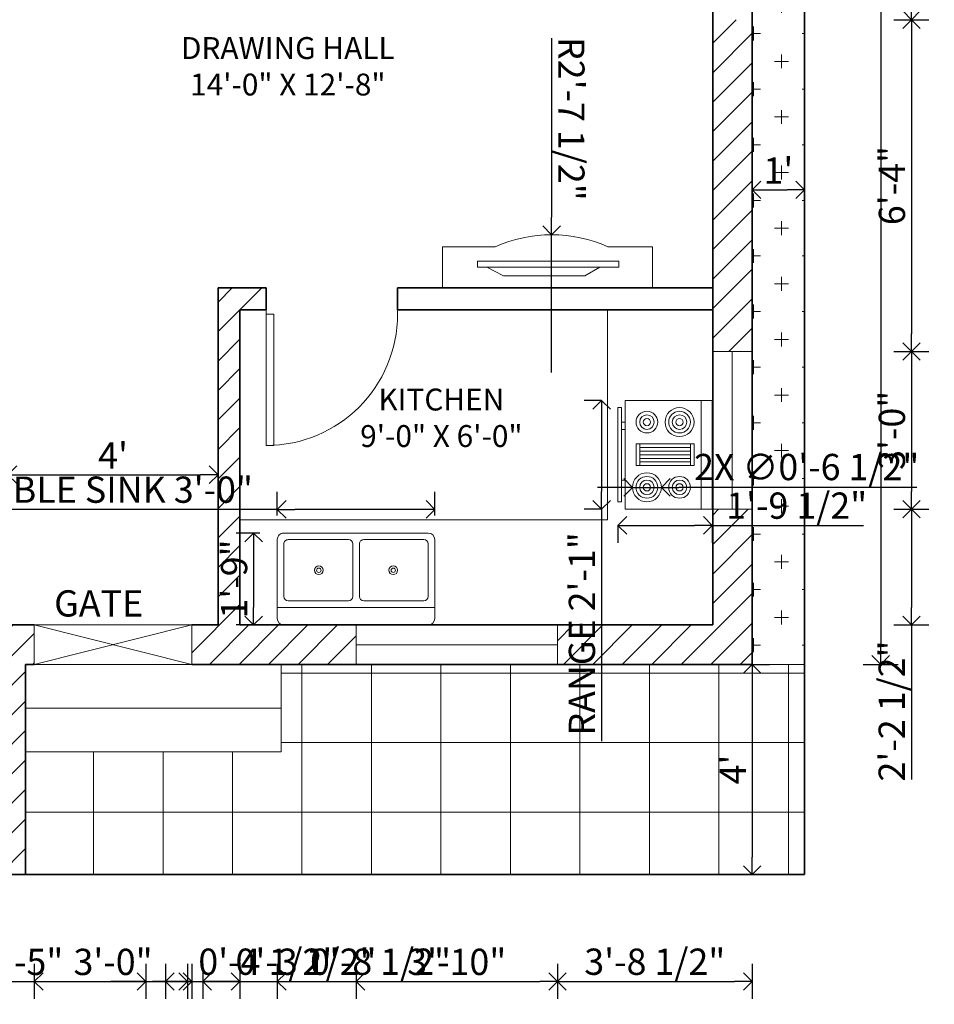
# Model space of a CAD drawing. Units: inches. Extents: x 686 to 1065, y 83 to 664.
# Tile 2 of 5: x 844 to 1053, y 83 to 308. Entities that reach past the tile are written whole.
import ezdxf

# ---------------------------------------------------------------- set-up
doc = ezdxf.new("R2010")
doc.units = ezdxf.units.IN
for name, color, linetype, lineweight in [('A-ANNO-DIMS', 2, 'Continuous', 18), ('A-ANNO-TEXT', 7, 'Continuous', 20), ('A-AREA-IDEN', 7, 'Continuous', 20), ('A-DOOR', 4, 'Continuous', 20), ('A-DOOR-GATE', 1, 'Continuous', 20), ('A-EQPM', 9, 'Continuous', 18), ('A-FLOR-CABN', 8, 'Continuous', 20), ('A-FLOR-FIXT', 9, 'Continuous', 18), ('A-FURN', 8, 'Continuous', 18), ('A-GLAZ', 172, 'Continuous', 18), ('A-WALL', 7, 'Continuous', 35), ('A-WALL-PATT', 253, 'Continuous', 13), ('C-PROP', 7, 'Continuous', 35), ('L-HRDS', 8, 'Continuous', 18), ('L-HRDS-PATT', 9, 'Continuous', 13), ('L-SITE-PATT', 94, 'Continuous', 13)]:
    doc.layers.add(name, color=color, linetype=linetype, lineweight=lineweight)
doc.styles.get("Standard").update_dxf_attribs({"font": 'arial.ttf'})
doc.dimstyles.new('ISO-25', dxfattribs={"dimtxt": 6, "dimasz": 4, "dimexe": 4, "dimexo": 4, "dimtad": 1, "dimdec": 1, "dimlunit": 3, "dimtxsty": 'Standard', "dimblk": 'OPEN90', "dimcen": 2.5, "dimadec": 0, "dimazin": 0, "dimtfac": 1, "dimtdec": 1, "dimtmove": 0, "dimatfit": 3, "dimfxl": 4, "dimfxlon": 1, "dimarcsym": 0})

# ---------------------------------------------------------------- blocks, each defined once
blk = doc.blocks.new('_Open90')
at = {"color": 0, "linetype": 'ByBlock', "lineweight": -2}
for p, q in [((0, 0), (-1, 0)), ((-0.5, 0.5), (0, 0)), ((0, 0), (-0.5, -0.5))]:
    blk.add_line(p, q, dxfattribs=at)
blk = doc.blocks.new('*D9')
at = {"layer": 'A-ANNO-DIMS', "color": 0, "lineweight": -2, "transparency": 16777216}
for p, q in [((1011.37, 265.11), (1011.37, 273.11)), ((1023.37, 265.11), (1023.37, 273.11)), ((1015.37, 269.11), (1019.37, 269.11))]:
    blk.add_line(p, q, dxfattribs=at)
at = {"layer": 'Defpoints', "color": 0, "transparency": 16777216}
for p in [(1023.37, 269.11), (1011.37, 160.73), (1023.37, 160.73)]:
    blk.add_point(p, dxfattribs=at)
at = {"layer": 'A-ANNO-DIMS', "color": 0, "lineweight": -2, "transparency": 16777216, "xscale": 4, "yscale": 4, "zscale": 4, "rotation": 180}
blk.add_blockref('_Open90', (1011.37, 269.11), dxfattribs=at)
at = {"layer": 'A-ANNO-DIMS', "color": 0, "lineweight": -2, "transparency": 16777216, "xscale": 4, "yscale": 4, "zscale": 4}
blk.add_blockref('_Open90', (1023.37, 269.11), dxfattribs=at)
at = {"layer": 'A-ANNO-DIMS', "color": 0, "transparency": 16777216, "insert": (1017.37, 272.75), "char_height": 6, "attachment_point": 5}
blk.add_mtext("1'", dxfattribs=at)
blk = doc.blocks.new('Range-Oven - 30 in top')
for p, q in [((0, -3), (30, -3)), ((12, -6), (18, -6)), ((13, -20), (13, -6)), ((14, -6), (14, -20)), ((15, -20), (15, -6)), ((16, -6), (16, -20)), ((17, -20), (17, -6)), ((18, -20), (12, -20)), ((6, -24), (6, -25)), ((8, -25), (8, -24)), ((22, -25), (22, -24)), ((24, -24), (24, -25))]:
    blk.add_line(p, q)
for points in [[(0, -24), (0, 0), (30, 0), (30, -24)], [(12, -21), (12, -5), (18, -5), (18, -21)], [(2, -26), (2, -25), (28, -25), (28, -26)]]:
    blk.add_lwpolyline(points, close=True)
for centre, radius in [((6, -9), 4), ((6, -9), 3), ((6, -9), 2), ((6, -9), 1), ((24, -9), 3), ((24, -9), 2), ((24, -9), 1), ((6, -18), 3), ((6, -18), 2), ((24, -18), 4), ((24, -18), 3), ((24, -18), 2), ((6, -18), 1), ((24, -18), 1)]:
    blk.add_circle(centre, radius)
blk = doc.blocks.new('Sink-double - 36 in top')
for p, q in [((-18, -4), (18, -4)), ((-0.75, -18.5), (-0.75, -6.5)), ((0.75, -6.5), (0.75, -18.5))]:
    blk.add_line(p, q)
for points in [[(-16.5, 0), (16.5, 0)], [(-18, -19.5), (-18, -1.5)], [(18, -1.5), (18, -19.5)], [(-16.5, -18.5), (-16.5, -6.5)], [(-15.5, -5.5), (-1.75, -5.5)], [(1.75, -5.5), (15.5, -5.5)], [(16.5, -6.5), (16.5, -18.5)], [(-1.75, -19.5), (-15.5, -19.5)], [(15.5, -19.5), (1.75, -19.5)], [(16.5, -21), (-16.5, -21)]]:
    blk.add_lwpolyline(points)
for centre, radius in [((-8.5, -12.5), 1), ((-8.5, -12.5), 0.5), ((8.5, -12.5), 1), ((8.5, -12.5), 0.5)]:
    blk.add_circle(centre, radius)
for centre, radius, start, end in [((-16.5, -1.5), 1.5, 90, 180), ((16.5, -1.5), 1.5, 0, 90), ((-15.5, -6.5), 1, 90, 180), ((-1.75, -6.5), 1, 0, 90), ((1.75, -6.5), 1, 90, 180), ((15.5, -6.5), 1, 0, 90), ((-16.5, -19.5), 1.5, 180, 270), ((-15.5, -18.5), 1, 180, 270), ((-1.75, -18.5), 1, 270, 0), ((1.75, -18.5), 1, 180, 270), ((15.5, -18.5), 1, 270, 0), ((16.5, -19.5), 1.5, 270, 0)]:
    blk.add_arc(centre, radius, start, end)
blk = doc.blocks.new('*D19')
at = {"layer": 'A-ANNO-DIMS', "color": 0, "lineweight": -2, "transparency": 16777216}
for p, q in [((841.37, 203.96), (841.37, 208.06)), ((889.37, 203.96), (889.37, 208.06)), ((845.37, 204.06), (885.37, 204.06))]:
    blk.add_line(p, q, dxfattribs=at)
at = {"layer": 'Defpoints', "color": 0, "transparency": 16777216}
for p in [(889.37, 204.06), (841.37, 199.96), (889.37, 199.96)]:
    blk.add_point(p, dxfattribs=at)
at = {"layer": 'A-ANNO-DIMS', "color": 0, "lineweight": -2, "transparency": 16777216, "xscale": 4, "yscale": 4, "zscale": 4, "rotation": 180}
blk.add_blockref('_Open90', (841.37, 204.06), dxfattribs=at)
at = {"layer": 'A-ANNO-DIMS', "color": 0, "lineweight": -2, "transparency": 16777216, "xscale": 4, "yscale": 4, "zscale": 4}
blk.add_blockref('_Open90', (889.37, 204.06), dxfattribs=at)
at = {"layer": 'A-ANNO-DIMS', "color": 0, "transparency": 16777216, "insert": (865.37, 207.68), "char_height": 6, "attachment_point": 5}
blk.add_mtext("4'", dxfattribs=at)
blk = doc.blocks.new('*D8')
at = {"layer": 'A-ANNO-DIMS', "color": 0, "lineweight": -2, "transparency": 16777216}
for p, q in [((1036.76, 592.73), (1044.76, 592.73)), ((1040.76, 588.73), (1040.76, 164.73)), ((1036.76, 160.73), (1044.76, 160.73))]:
    blk.add_line(p, q, dxfattribs=at)
at = {"layer": 'Defpoints', "color": 0, "transparency": 16777216}
for p in [(1023.37, 592.73), (1023.37, 160.73), (1040.76, 160.73)]:
    blk.add_point(p, dxfattribs=at)
at = {"layer": 'A-ANNO-DIMS', "color": 0, "lineweight": -2, "transparency": 16777216, "xscale": 4, "yscale": 4, "zscale": 4}
for p, rotation in [((1040.76, 592.73), 90), ((1040.76, 160.73), 270)]:
    blk.add_blockref('_Open90', p, dxfattribs=dict(at, rotation=rotation))
at = {"layer": 'A-ANNO-DIMS', "color": 0, "transparency": 16777216, "insert": (1037.07, 376.73), "char_height": 6, "attachment_point": 5, "rotation": 90}
blk.add_mtext("36'", dxfattribs=at)
blk = doc.blocks.new('*D20')
at = {"layer": 'A-ANNO-DIMS', "color": 0, "lineweight": -2, "transparency": 16777216}
for p, q in [((1011.37, 160.73), (1015.37, 160.73)), ((1011.37, 156.73), (1011.37, 116.73)), ((1011.37, 112.73), (1015.37, 112.73))]:
    blk.add_line(p, q, dxfattribs=at)
at = {"layer": 'Defpoints', "color": 0, "transparency": 16777216}
for p in [(1011.37, 160.73), (1011.37, 112.73), (1011.37, 112.73)]:
    blk.add_point(p, dxfattribs=at)
at = {"layer": 'A-ANNO-DIMS', "color": 0, "lineweight": -2, "transparency": 16777216, "xscale": 4, "yscale": 4, "zscale": 4}
for p, rotation in [((1011.37, 160.73), 90), ((1011.37, 112.73), 270)]:
    blk.add_blockref('_Open90', p, dxfattribs=dict(at, rotation=rotation))
at = {"layer": 'A-ANNO-DIMS', "color": 0, "transparency": 16777216, "insert": (1007.75, 136.73), "char_height": 6, "attachment_point": 5, "rotation": 90}
blk.add_mtext("4'", dxfattribs=at)
blk = doc.blocks.new('*U24')
for p, q in [((-30, 0), (-30, -6)), ((0, 0), (0, -6))]:
    blk.add_line(p, q)
blk.add_lwpolyline([(0, 0), (0, 30), (-1.75, 30), (-1.75, 0)], close=True)
blk.add_arc((0, 0), 30, 90, 180)
blk = doc.blocks.new('*D32')
at = {"layer": 'A-ANNO-DIMS', "color": 0, "lineweight": -2, "transparency": 16777216}
for p, q in [((977, 221.04), (973, 221.04)), ((977, 217.04), (977, 200.2)), ((977, 196.2), (973, 196.2)), ((977, 196.2), (977, 143.18))]:
    blk.add_line(p, q, dxfattribs=at)
at = {"layer": 'Defpoints', "color": 0, "transparency": 16777216}
for p in [(980.72, 221.04), (977, 196.2), (980.72, 196.2)]:
    blk.add_point(p, dxfattribs=at)
at = {"layer": 'A-ANNO-DIMS', "color": 0, "lineweight": -2, "transparency": 16777216, "xscale": 4, "yscale": 4, "zscale": 4}
for p, rotation in [((977, 221.04), 90), ((977, 196.2), 270)]:
    blk.add_blockref('_Open90', p, dxfattribs=dict(at, rotation=rotation))
at = {"layer": 'A-ANNO-DIMS', "color": 0, "transparency": 16777216, "insert": (973.27, 167.69), "char_height": 6, "attachment_point": 5, "rotation": 90}
blk.add_mtext('RANGE 2\'-1"', dxfattribs=at)
blk = doc.blocks.new('*D33')
at = {"layer": 'A-ANNO-DIMS', "color": 0, "lineweight": -2, "transparency": 16777216}
for p, q in [((980.72, 192.48), (980.72, 188.48)), ((984.72, 192.48), (998.25, 192.48)), ((1002.25, 192.48), (1002.25, 188.48)), ((1002.25, 192.48), (1036.86, 192.48))]:
    blk.add_line(p, q, dxfattribs=at)
at = {"layer": 'Defpoints', "color": 0, "transparency": 16777216}
for p in [(980.72, 196.2), (1002.25, 196.2), (1002.25, 192.48)]:
    blk.add_point(p, dxfattribs=at)
at = {"layer": 'A-ANNO-DIMS', "color": 0, "lineweight": -2, "transparency": 16777216, "xscale": 4, "yscale": 4, "zscale": 4, "rotation": 180}
blk.add_blockref('_Open90', (980.72, 192.48), dxfattribs=at)
at = {"layer": 'A-ANNO-DIMS', "color": 0, "lineweight": -2, "transparency": 16777216, "xscale": 4, "yscale": 4, "zscale": 4}
blk.add_blockref('_Open90', (1002.25, 192.48), dxfattribs=at)
at = {"layer": 'A-ANNO-DIMS', "color": 0, "transparency": 16777216, "insert": (1021.56, 196.21), "char_height": 6, "attachment_point": 5}
blk.add_mtext('1\'-9 1/2"', dxfattribs=at)
blk = doc.blocks.new('*D40')
at = {"layer": 'A-ANNO-DIMS', "color": 0, "lineweight": -2, "transparency": 16777216}
for p, q in [((902.89, 194.73), (902.89, 200.13)), ((938.89, 194.73), (938.89, 200.13)), ((902.89, 196.13), (823.3, 196.13)), ((934.89, 196.13), (906.89, 196.13))]:
    blk.add_line(p, q, dxfattribs=at)
at = {"layer": 'Defpoints', "color": 0, "transparency": 16777216}
for p in [(902.89, 196.13), (902.89, 190.73), (938.89, 190.73)]:
    blk.add_point(p, dxfattribs=at)
at = {"layer": 'A-ANNO-DIMS', "color": 0, "lineweight": -2, "transparency": 16777216, "xscale": 4, "yscale": 4, "zscale": 4, "rotation": 180}
blk.add_blockref('_Open90', (902.89, 196.13), dxfattribs=at)
at = {"layer": 'A-ANNO-DIMS', "color": 0, "lineweight": -2, "transparency": 16777216, "xscale": 4, "yscale": 4, "zscale": 4}
blk.add_blockref('_Open90', (938.89, 196.13), dxfattribs=at)
at = {"layer": 'A-ANNO-DIMS', "color": 0, "transparency": 16777216, "insert": (861.09, 199.86), "char_height": 6, "attachment_point": 5}
blk.add_mtext('DOUBLE SINK 3\'-0"', dxfattribs=at)
blk = doc.blocks.new('*D41')
at = {"layer": 'A-ANNO-DIMS', "color": 0, "lineweight": -2, "transparency": 16777216}
for p, q in [((898.89, 190.73), (893.49, 190.73)), ((897.49, 186.73), (897.49, 173.73)), ((898.89, 169.73), (893.49, 169.73))]:
    blk.add_line(p, q, dxfattribs=at)
at = {"layer": 'Defpoints', "color": 0, "transparency": 16777216}
for p in [(902.89, 190.73), (897.49, 169.73), (902.89, 169.73)]:
    blk.add_point(p, dxfattribs=at)
at = {"layer": 'A-ANNO-DIMS', "color": 0, "lineweight": -2, "transparency": 16777216, "xscale": 4, "yscale": 4, "zscale": 4}
for p, rotation in [((897.49, 190.73), 90), ((897.49, 169.73), 270)]:
    blk.add_blockref('_Open90', p, dxfattribs=dict(at, rotation=rotation))
at = {"layer": 'A-ANNO-DIMS', "color": 0, "transparency": 16777216, "insert": (893.8, 180.23), "char_height": 6, "attachment_point": 5, "rotation": 90}
blk.add_mtext('1\'-9"', dxfattribs=at)
blk = doc.blocks.new('*D49')
at = {"layer": 'A-ANNO-DIMS', "color": 0, "lineweight": -2, "transparency": 16777216}
for p, q in [((1043.78, 363.95), (1051.78, 363.95)), ((1047.78, 359.95), (1047.78, 311.98)), ((1043.78, 307.98), (1051.78, 307.98))]:
    blk.add_line(p, q, dxfattribs=at)
at = {"layer": 'Defpoints', "color": 0, "transparency": 16777216}
for p in [(1011.37, 363.95), (1011.37, 307.98), (1047.78, 307.98)]:
    blk.add_point(p, dxfattribs=at)
at = {"layer": 'A-ANNO-DIMS', "color": 0, "lineweight": -2, "transparency": 16777216, "xscale": 4, "yscale": 4, "zscale": 4}
for p, rotation in [((1047.78, 363.95), 90), ((1047.78, 307.98), 270)]:
    blk.add_blockref('_Open90', p, dxfattribs=dict(at, rotation=rotation))
at = {"layer": 'A-ANNO-DIMS', "color": 0, "transparency": 16777216, "insert": (1044.09, 335.96), "char_height": 6, "attachment_point": 5, "rotation": 90}
blk.add_mtext('4\'-8"', dxfattribs=at)
blk = doc.blocks.new('*D50')
at = {"layer": 'A-ANNO-DIMS', "color": 0, "lineweight": -2, "transparency": 16777216}
for p, q in [((1043.78, 307.98), (1051.78, 307.98)), ((1047.78, 303.98), (1047.78, 236.2)), ((1043.78, 232.2), (1051.78, 232.2))]:
    blk.add_line(p, q, dxfattribs=at)
at = {"layer": 'Defpoints', "color": 0, "transparency": 16777216}
for p in [(1011.37, 307.98), (1011.37, 232.2), (1047.78, 232.2)]:
    blk.add_point(p, dxfattribs=at)
at = {"layer": 'A-ANNO-DIMS', "color": 0, "lineweight": -2, "transparency": 16777216, "xscale": 4, "yscale": 4, "zscale": 4}
for p, rotation in [((1047.78, 307.98), 90), ((1047.78, 232.2), 270)]:
    blk.add_blockref('_Open90', p, dxfattribs=dict(at, rotation=rotation))
at = {"layer": 'A-ANNO-DIMS', "color": 0, "transparency": 16777216, "insert": (1044.09, 270.09), "char_height": 6, "attachment_point": 5, "rotation": 90}
blk.add_mtext('6\'-4"', dxfattribs=at)
blk = doc.blocks.new('*D51')
at = {"layer": 'A-ANNO-DIMS', "color": 0, "lineweight": -2, "transparency": 16777216}
for p, q in [((1043.78, 232.2), (1051.78, 232.2)), ((1047.78, 228.2), (1047.78, 200.2)), ((1043.78, 196.2), (1051.78, 196.2))]:
    blk.add_line(p, q, dxfattribs=at)
at = {"layer": 'Defpoints', "color": 0, "transparency": 16777216}
for p in [(1011.37, 232.2), (1011.37, 196.2), (1047.78, 196.2)]:
    blk.add_point(p, dxfattribs=at)
at = {"layer": 'A-ANNO-DIMS', "color": 0, "lineweight": -2, "transparency": 16777216, "xscale": 4, "yscale": 4, "zscale": 4}
for p, rotation in [((1047.78, 232.2), 90), ((1047.78, 196.2), 270)]:
    blk.add_blockref('_Open90', p, dxfattribs=dict(at, rotation=rotation))
at = {"layer": 'A-ANNO-DIMS', "color": 0, "transparency": 16777216, "insert": (1044.09, 214.2), "char_height": 6, "attachment_point": 5, "rotation": 90}
blk.add_mtext('3\'-0"', dxfattribs=at)
blk = doc.blocks.new('*D52')
at = {"layer": 'A-ANNO-DIMS', "color": 0, "lineweight": -2, "transparency": 16777216}
for p, q in [((920.89, 92.32), (920.89, 84.32)), ((966.91, 92.32), (966.91, 84.32)), ((924.89, 88.32), (962.91, 88.32))]:
    blk.add_line(p, q, dxfattribs=at)
at = {"layer": 'Defpoints', "color": 0, "transparency": 16777216}
for p in [(920.89, 160.73), (966.91, 160.73), (966.91, 88.32)]:
    blk.add_point(p, dxfattribs=at)
at = {"layer": 'A-ANNO-DIMS', "color": 0, "lineweight": -2, "transparency": 16777216, "xscale": 4, "yscale": 4, "zscale": 4, "rotation": 180}
blk.add_blockref('_Open90', (920.89, 88.32), dxfattribs=at)
at = {"layer": 'A-ANNO-DIMS', "color": 0, "lineweight": -2, "transparency": 16777216, "xscale": 4, "yscale": 4, "zscale": 4}
blk.add_blockref('_Open90', (966.91, 88.32), dxfattribs=at)
at = {"layer": 'A-ANNO-DIMS', "color": 0, "transparency": 16777216, "insert": (943.9, 92.01), "char_height": 6, "attachment_point": 5}
blk.add_mtext('3\'-10"', dxfattribs=at)
blk = doc.blocks.new('*D53')
at = {"layer": 'A-ANNO-DIMS', "color": 0, "lineweight": -2, "transparency": 16777216}
for p, q in [((966.91, 92.32), (966.91, 84.32)), ((1011.37, 92.32), (1011.37, 84.32)), ((970.91, 88.32), (1007.37, 88.32))]:
    blk.add_line(p, q, dxfattribs=at)
at = {"layer": 'Defpoints', "color": 0, "transparency": 16777216}
for p in [(966.91, 160.73), (1011.37, 160.73), (1011.37, 88.32)]:
    blk.add_point(p, dxfattribs=at)
at = {"layer": 'A-ANNO-DIMS', "color": 0, "lineweight": -2, "transparency": 16777216, "xscale": 4, "yscale": 4, "zscale": 4, "rotation": 180}
blk.add_blockref('_Open90', (966.91, 88.32), dxfattribs=at)
at = {"layer": 'A-ANNO-DIMS', "color": 0, "lineweight": -2, "transparency": 16777216, "xscale": 4, "yscale": 4, "zscale": 4}
blk.add_blockref('_Open90', (1011.37, 88.32), dxfattribs=at)
at = {"layer": 'A-ANNO-DIMS', "color": 0, "transparency": 16777216, "insert": (989.14, 92.05), "char_height": 6, "attachment_point": 5}
blk.add_mtext('3\'-8 1/2"', dxfattribs=at)
blk = doc.blocks.new('*D56')
at = {"layer": 'A-ANNO-DIMS', "color": 0, "lineweight": -2, "transparency": 16777216}
for p, q in [((900.37, 613.14), (900.37, 621.14)), ((930.37, 613.14), (930.37, 621.14)), ((904.37, 617.14), (926.37, 617.14))]:
    blk.add_line(p, q, dxfattribs=at)
at = {"layer": 'Defpoints', "color": 0, "transparency": 16777216}
for p in [(930.37, 617.14), (900.37, 246.73), (930.37, 246.73)]:
    blk.add_point(p, dxfattribs=at)
at = {"layer": 'A-ANNO-DIMS', "color": 0, "lineweight": -2, "transparency": 16777216, "xscale": 4, "yscale": 4, "zscale": 4, "rotation": 180}
blk.add_blockref('_Open90', (900.37, 617.14), dxfattribs=at)
at = {"layer": 'A-ANNO-DIMS', "color": 0, "lineweight": -2, "transparency": 16777216, "xscale": 4, "yscale": 4, "zscale": 4}
blk.add_blockref('_Open90', (930.37, 617.14), dxfattribs=at)
at = {"layer": 'A-ANNO-DIMS', "color": 0, "transparency": 16777216, "insert": (915.37, 620.83), "char_height": 6, "attachment_point": 5}
blk.add_mtext('2\'-6"', dxfattribs=at)
blk = doc.blocks.new('*D58')
at = {"layer": 'A-ANNO-DIMS', "color": 0, "lineweight": -2, "transparency": 16777216}
for p, q in [((847.37, 92.32), (847.37, 84.32)), ((883.37, 92.32), (883.37, 84.32)), ((851.37, 88.32), (879.37, 88.32))]:
    blk.add_line(p, q, dxfattribs=at)
at = {"layer": 'Defpoints', "color": 0, "transparency": 16777216}
for p in [(847.37, 160.73), (883.37, 160.73), (883.37, 88.32)]:
    blk.add_point(p, dxfattribs=at)
at = {"layer": 'A-ANNO-DIMS', "color": 0, "lineweight": -2, "transparency": 16777216, "xscale": 4, "yscale": 4, "zscale": 4, "rotation": 180}
blk.add_blockref('_Open90', (847.37, 88.32), dxfattribs=at)
at = {"layer": 'A-ANNO-DIMS', "color": 0, "lineweight": -2, "transparency": 16777216, "xscale": 4, "yscale": 4, "zscale": 4}
blk.add_blockref('_Open90', (883.37, 88.32), dxfattribs=at)
at = {"layer": 'A-ANNO-DIMS', "color": 0, "transparency": 16777216, "insert": (865.37, 92.01), "char_height": 6, "attachment_point": 5}
blk.add_mtext('3\'-0"', dxfattribs=at)
blk = doc.blocks.new('*D63')
at = {"layer": 'A-ANNO-DIMS', "color": 0, "lineweight": -2, "transparency": 16777216}
for p, q in [((823.37, 92.32), (823.37, 84.32)), ((828.37, 92.32), (828.37, 84.32)), ((819.37, 88.32), (815.37, 88.32)), ((823.37, 88.32), (828.37, 88.32)), ((832.37, 88.32), (853.57, 88.32))]:
    blk.add_line(p, q, dxfattribs=at)
at = {"layer": 'Defpoints', "color": 0, "transparency": 16777216}
for p in [(823.37, 362.73), (828.37, 357.73), (828.37, 88.32)]:
    blk.add_point(p, dxfattribs=at)
at = {"layer": 'A-ANNO-DIMS', "color": 0, "lineweight": -2, "transparency": 16777216, "xscale": 4, "yscale": 4, "zscale": 4}
blk.add_blockref('_Open90', (823.37, 88.32), dxfattribs=at)
at = {"layer": 'A-ANNO-DIMS', "color": 0, "lineweight": -2, "transparency": 16777216, "xscale": 4, "yscale": 4, "zscale": 4, "rotation": 180}
blk.add_blockref('_Open90', (828.37, 88.32), dxfattribs=at)
at = {"layer": 'A-ANNO-DIMS', "color": 0, "transparency": 16777216, "insert": (844.97, 92.01), "char_height": 6, "attachment_point": 5}
blk.add_mtext('0\'-5"', dxfattribs=at)
blk = doc.blocks.new('*D64')
at = {"layer": 'A-ANNO-DIMS', "color": 0, "lineweight": -2, "transparency": 16777216}
for p, q in [((872.87, 92.32), (872.87, 84.32)), ((877.37, 92.32), (877.37, 84.32)), ((868.87, 88.32), (864.87, 88.32)), ((872.87, 88.32), (877.37, 88.32)), ((881.37, 88.32), (916.55, 88.32))]:
    blk.add_line(p, q, dxfattribs=at)
at = {"layer": 'Defpoints', "color": 0, "transparency": 16777216}
for p in [(877.37, 415.73), (872.87, 410.73), (877.37, 88.32)]:
    blk.add_point(p, dxfattribs=at)
at = {"layer": 'A-ANNO-DIMS', "color": 0, "lineweight": -2, "transparency": 16777216, "xscale": 4, "yscale": 4, "zscale": 4}
blk.add_blockref('_Open90', (872.87, 88.32), dxfattribs=at)
at = {"layer": 'A-ANNO-DIMS', "color": 0, "lineweight": -2, "transparency": 16777216, "xscale": 4, "yscale": 4, "zscale": 4, "rotation": 180}
blk.add_blockref('_Open90', (877.37, 88.32), dxfattribs=at)
at = {"layer": 'A-ANNO-DIMS', "color": 0, "transparency": 16777216, "insert": (900.96, 92.05), "char_height": 6, "attachment_point": 5}
blk.add_mtext('0\'-4 1/2"', dxfattribs=at)
blk = doc.blocks.new('*D65')
at = {"layer": 'A-ANNO-DIMS', "color": 0, "lineweight": -2, "transparency": 16777216}
for p, q in [((882.37, 92.32), (882.37, 84.32)), ((885.87, 92.32), (885.87, 84.32)), ((878.37, 88.32), (874.37, 88.32)), ((882.37, 88.32), (885.87, 88.32)), ((889.87, 88.32), (925.05, 88.32))]:
    blk.add_line(p, q, dxfattribs=at)
at = {"layer": 'Defpoints', "color": 0, "transparency": 16777216}
for p in [(882.37, 415.73), (885.87, 410.73), (885.87, 88.32)]:
    blk.add_point(p, dxfattribs=at)
at = {"layer": 'A-ANNO-DIMS', "color": 0, "lineweight": -2, "transparency": 16777216, "xscale": 4, "yscale": 4, "zscale": 4}
blk.add_blockref('_Open90', (882.37, 88.32), dxfattribs=at)
at = {"layer": 'A-ANNO-DIMS', "color": 0, "lineweight": -2, "transparency": 16777216, "xscale": 4, "yscale": 4, "zscale": 4, "rotation": 180}
blk.add_blockref('_Open90', (885.87, 88.32), dxfattribs=at)
at = {"layer": 'A-ANNO-DIMS', "color": 0, "transparency": 16777216, "insert": (909.46, 92.05), "char_height": 6, "attachment_point": 5}
blk.add_mtext('0\'-3 1/2"', dxfattribs=at)
blk = doc.blocks.new('*D66')
at = {"layer": 'A-ANNO-DIMS', "color": 0, "lineweight": -2, "transparency": 16777216}
for p, q in [((894.37, 613.14), (894.37, 621.14)), ((900.37, 613.14), (900.37, 621.14)), ((890.37, 617.14), (886.37, 617.14)), ((894.37, 617.14), (900.37, 617.14)), ((904.37, 617.14), (925.57, 617.14))]:
    blk.add_line(p, q, dxfattribs=at)
at = {"layer": 'Defpoints', "color": 0, "transparency": 16777216}
for p in [(900.37, 617.14), (894.37, 241.73), (900.37, 241.73)]:
    blk.add_point(p, dxfattribs=at)
at = {"layer": 'A-ANNO-DIMS', "color": 0, "lineweight": -2, "transparency": 16777216, "xscale": 4, "yscale": 4, "zscale": 4}
blk.add_blockref('_Open90', (894.37, 617.14), dxfattribs=at)
at = {"layer": 'A-ANNO-DIMS', "color": 0, "lineweight": -2, "transparency": 16777216, "xscale": 4, "yscale": 4, "zscale": 4, "rotation": 180}
blk.add_blockref('_Open90', (900.37, 617.14), dxfattribs=at)
at = {"layer": 'A-ANNO-DIMS', "color": 0, "transparency": 16777216, "insert": (916.97, 620.83), "char_height": 6, "attachment_point": 5}
blk.add_mtext('0\'-6"', dxfattribs=at)
blk = doc.blocks.new('*D69')
at = {"layer": 'A-ANNO-DIMS', "color": 0, "lineweight": -2, "transparency": 16777216}
for p, q in [((978.37, 613.14), (978.37, 621.14)), ((1002.37, 613.14), (1002.37, 621.14)), ((982.37, 617.14), (998.37, 617.14))]:
    blk.add_line(p, q, dxfattribs=at)
at = {"layer": 'Defpoints', "color": 0, "transparency": 16777216}
for p in [(1002.37, 617.14), (978.37, 241.73), (1002.37, 241.73)]:
    blk.add_point(p, dxfattribs=at)
at = {"layer": 'A-ANNO-DIMS', "color": 0, "lineweight": -2, "transparency": 16777216, "xscale": 4, "yscale": 4, "zscale": 4, "rotation": 180}
blk.add_blockref('_Open90', (978.37, 617.14), dxfattribs=at)
at = {"layer": 'A-ANNO-DIMS', "color": 0, "lineweight": -2, "transparency": 16777216, "xscale": 4, "yscale": 4, "zscale": 4}
blk.add_blockref('_Open90', (1002.37, 617.14), dxfattribs=at)
at = {"layer": 'A-ANNO-DIMS', "color": 0, "transparency": 16777216, "insert": (990.37, 620.83), "char_height": 6, "attachment_point": 5}
blk.add_mtext('2\'-0"', dxfattribs=at)
blk = doc.blocks.new('*D70')
at = {"layer": 'A-ANNO-DIMS', "color": 0, "lineweight": -2, "transparency": 16777216}
for p, q in [((702.96, 193.73), (694.96, 193.73)), ((698.96, 173.73), (698.96, 189.73)), ((702.96, 169.73), (694.96, 169.73))]:
    blk.add_line(p, q, dxfattribs=at)
at = {"layer": 'Defpoints', "color": 0, "transparency": 16777216}
for p in [(698.96, 193.73), (894.37, 193.73), (894.37, 169.73)]:
    blk.add_point(p, dxfattribs=at)
at = {"layer": 'A-ANNO-DIMS', "color": 0, "lineweight": -2, "transparency": 16777216, "xscale": 4, "yscale": 4, "zscale": 4}
for p, rotation in [((698.96, 193.73), 90), ((698.96, 169.73), 270)]:
    blk.add_blockref('_Open90', p, dxfattribs=dict(at, rotation=rotation))
at = {"layer": 'A-ANNO-DIMS', "color": 0, "transparency": 16777216, "insert": (695.27, 181.73), "char_height": 6, "attachment_point": 5, "rotation": 90}
blk.add_mtext('2\'-0"', dxfattribs=at)
blk = doc.blocks.new('*D71')
at = {"layer": 'A-ANNO-DIMS', "color": 0, "lineweight": -2, "transparency": 16777216}
for p, q in [((894.37, 92.32), (894.37, 84.32)), ((902.89, 92.32), (902.89, 84.32)), ((890.37, 88.32), (886.37, 88.32)), ((894.37, 88.32), (902.89, 88.32)), ((906.89, 88.32), (942.07, 88.32))]:
    blk.add_line(p, q, dxfattribs=at)
at = {"layer": 'Defpoints', "color": 0, "transparency": 16777216}
for p in [(902.89, 173.73), (894.37, 169.73), (902.89, 88.32)]:
    blk.add_point(p, dxfattribs=at)
at = {"layer": 'A-ANNO-DIMS', "color": 0, "lineweight": -2, "transparency": 16777216, "xscale": 4, "yscale": 4, "zscale": 4}
blk.add_blockref('_Open90', (894.37, 88.32), dxfattribs=at)
at = {"layer": 'A-ANNO-DIMS', "color": 0, "lineweight": -2, "transparency": 16777216, "xscale": 4, "yscale": 4, "zscale": 4, "rotation": 180}
blk.add_blockref('_Open90', (902.89, 88.32), dxfattribs=at)
at = {"layer": 'A-ANNO-DIMS', "color": 0, "transparency": 16777216, "insert": (926.48, 92.05), "char_height": 6, "attachment_point": 5}
blk.add_mtext('0\'-8 1/2"', dxfattribs=at)
blk = doc.blocks.new('*D72')
at = {"layer": 'A-ANNO-DIMS', "color": 0, "lineweight": -2, "transparency": 16777216}
for p, q in [((1043.78, 196.2), (1051.78, 196.2)), ((1047.78, 192.2), (1047.78, 173.73)), ((1043.78, 169.73), (1051.78, 169.73)), ((1047.78, 169.73), (1047.78, 134.45))]:
    blk.add_line(p, q, dxfattribs=at)
at = {"layer": 'Defpoints', "color": 0, "transparency": 16777216}
for p in [(1002.25, 196.2), (1002.37, 169.73), (1047.78, 169.73)]:
    blk.add_point(p, dxfattribs=at)
at = {"layer": 'A-ANNO-DIMS', "color": 0, "lineweight": -2, "transparency": 16777216, "xscale": 4, "yscale": 4, "zscale": 4}
for p, rotation in [((1047.78, 196.2), 90), ((1047.78, 169.73), 270)]:
    blk.add_blockref('_Open90', p, dxfattribs=dict(at, rotation=rotation))
at = {"layer": 'A-ANNO-DIMS', "color": 0, "transparency": 16777216, "insert": (1044.05, 150.09), "char_height": 6, "attachment_point": 5, "rotation": 90}
blk.add_mtext('2\'-2 1/2"', dxfattribs=at)
blk = doc.blocks.new('*D75')
at = {"layer": 'A-ANNO-DIMS', "color": 0, "lineweight": -2, "transparency": 16777216}
for p, q in [((841.37, 613.14), (841.37, 621.14)), ((847.37, 613.14), (847.37, 621.14)), ((837.37, 617.14), (833.37, 617.14)), ((841.37, 617.14), (847.37, 617.14)), ((851.37, 617.14), (872.57, 617.14))]:
    blk.add_line(p, q, dxfattribs=at)
at = {"layer": 'Defpoints', "color": 0, "transparency": 16777216}
for p in [(847.37, 617.14), (841.37, 169.73), (847.37, 169.73)]:
    blk.add_point(p, dxfattribs=at)
at = {"layer": 'A-ANNO-DIMS', "color": 0, "lineweight": -2, "transparency": 16777216, "xscale": 4, "yscale": 4, "zscale": 4}
blk.add_blockref('_Open90', (841.37, 617.14), dxfattribs=at)
at = {"layer": 'A-ANNO-DIMS', "color": 0, "lineweight": -2, "transparency": 16777216, "xscale": 4, "yscale": 4, "zscale": 4, "rotation": 180}
blk.add_blockref('_Open90', (847.37, 617.14), dxfattribs=at)
at = {"layer": 'A-ANNO-DIMS', "color": 0, "transparency": 16777216, "insert": (863.97, 620.83), "char_height": 6, "attachment_point": 5}
blk.add_mtext('0\'-6"', dxfattribs=at)
blk = doc.blocks.new('*D81')
at = {"layer": 'A-ANNO-DIMS', "color": 0, "lineweight": -2, "transparency": 16777216}
for p, q in [((965.58, 303.79), (965.58, 262.86)), ((965.58, 227.41), (965.58, 258.86))]:
    blk.add_line(p, q, dxfattribs=at)
at = {"layer": 'Defpoints', "color": 0, "transparency": 16777216}
for p in [(965.58, 258.86), (965.58, 227.41)]:
    blk.add_point(p, dxfattribs=at)
at = {"layer": 'A-ANNO-DIMS', "color": 0, "lineweight": -2, "transparency": 16777216, "xscale": 4, "yscale": 4, "zscale": 4, "rotation": 270.000533748316}
blk.add_blockref('_Open90', (965.58, 258.86), dxfattribs=at)
at = {"layer": 'A-ANNO-DIMS', "color": 0, "transparency": 16777216, "insert": (969.3, 285.33), "char_height": 6, "attachment_point": 5, "rotation": 270.0005}
blk.add_mtext('R2\'-7 1/2"', dxfattribs=at)
blk = doc.blocks.new('*D82')
at = {"layer": 'A-ANNO-DIMS', "color": 0, "lineweight": -2, "transparency": 16777216}
for p, q in [((980.03, 201.17), (976.03, 201.17)), ((984.03, 201.17), (990.66, 201.17)), ((1049.04, 201.17), (994.66, 201.17))]:
    blk.add_line(p, q, dxfattribs=at)
at = {"layer": 'Defpoints', "color": 0, "transparency": 16777216}
for p in [(984.03, 201.17), (990.66, 201.17)]:
    blk.add_point(p, dxfattribs=at)
at = {"layer": 'A-ANNO-DIMS', "color": 0, "lineweight": -2, "transparency": 16777216, "xscale": 4, "yscale": 4, "zscale": 4}
for p, rotation in [((984.03, 201.17), 359.9994290698719), ((990.66, 201.17), 179.9994290698719)]:
    blk.add_blockref('_Open90', p, dxfattribs=dict(at, rotation=rotation))
at = {"layer": 'A-ANNO-DIMS', "color": 0, "transparency": 16777216, "insert": (1023.85, 205.03), "char_height": 6, "attachment_point": 5, "rotation": 359.9994}
blk.add_mtext('2X ∅0\'-6 1/2"', dxfattribs=at)

msp = doc.modelspace()

# ---------------------------------------------------------------- hatches: boundary and pattern name
at = {"layer": 'A-WALL-PATT'}
h = msp.add_hatch(dxfattribs=at)
h.set_pattern_fill('ANSI31', color=256, scale=1.5)
h.set_pattern_definition([(45, (464.028, 0), (-3.367596, 3.367596), [])])
h.paths.add_polyline_path([(1011.37, 568.73), (742.37, 568.73), (742.37, 499.41), (751.37, 499.41), (751.37, 559.73), (877.37, 559.73), (877.37, 415.73), (872.87, 415.73), (872.87, 410.73), (885.87, 410.73), (885.87, 415.73), (882.37, 415.73), (882.37, 559.73), (1002.37, 559.73), (1002.37, 514.56), (1011.37, 514.56)])
h.paths.add_polyline_path([(832.87, 415.73), (751.37, 415.73), (751.37, 448.47), (742.37, 448.47), (742.37, 397.23), (751.37, 397.23), (751.37, 410.73), (823.37, 410.73), (823.37, 404.73), (828.37, 404.73), (828.37, 410.73), (832.87, 410.73)])
h.paths.add_polyline_path([(751.37, 357.73), (828.37, 357.73), (828.37, 372.73), (823.37, 372.73), (823.37, 362.73), (751.37, 362.73), (751.37, 376.23), (742.37, 376.23), (742.37, 112.73), (751.37, 112.73)])
h.paths.add_polyline_path([(845.37, 160.73), (847.37, 160.73), (847.37, 169.73), (841.37, 169.73), (841.37, 246.73), (836.37, 246.73), (836.37, 117.73), (807.43, 117.73), (807.43, 112.73), (845.37, 112.73)])
h.paths.add_polyline_path([(920.89, 169.73), (904.39, 169.73), (894.37, 169.73), (894.37, 241.73), (900.37, 241.73), (900.37, 246.73), (889.37, 246.73), (889.37, 169.73), (883.37, 169.73), (883.37, 160.73), (920.89, 160.73)])
h.paths.add_polyline_path([(1011.37, 196.2), (1002.37, 196.2), (1002.37, 169.73), (966.91, 169.73), (966.91, 160.73), (1011.37, 160.73)])
h.paths.add_polyline_path([(1011.37, 307.98), (1002.37, 307.98), (1002.37, 232.2), (1011.37, 232.2)])
h.paths.add_polyline_path([(1011.37, 463.11), (1002.37, 463.11), (1002.37, 415.73), (921.87, 415.73), (921.87, 410.73), (1002.37, 410.73), (1002.37, 363.95), (1011.37, 363.95)])
h.paths.add_polyline_path([(781.1, 117.73), (751.37, 117.73), (751.37, 112.73), (781.1, 112.73)], flags=17)
at = {"layer": 'L-HRDS-PATT'}
h = msp.add_hatch(dxfattribs=at)
h.set_pattern_fill('ANSI31', color=256, scale=5, angle=45)
h.set_pattern_definition([(90, (464.028, 0), (-15.875, 0), [])])
h.paths.add_polyline_path([(903.76, 160.73), (903.76, 140.73), (845.37, 140.73), (845.37, 112.73), (1023.37, 112.73), (1023.37, 160.73), (1011.37, 160.73)])
h = msp.add_hatch(dxfattribs=at)
h.set_pattern_fill('ANSI31', color=256, scale=5, angle=135)
h.set_pattern_definition([(180, (464.028, 0), (-2e-15, -15.875), [])])
h.paths.add_polyline_path([(1023.37, 112.73), (1023.37, 160.73), (1011.37, 160.73), (903.76, 160.73), (903.76, 140.73), (845.37, 140.73), (845.37, 112.73)])
at = {"layer": 'L-SITE-PATT'}
h = msp.add_hatch(dxfattribs=at)
h.set_pattern_fill('CROSS', color=256)
h.set_pattern_definition([(0, (464.028, 0), (6.35, 6.35), [3.175, -9.525]), (90, (465.6154, -1.5875), (-6.35, 6.35), [3.175, -9.525])])
h.paths.add_polyline_path([(742.37, 568.73), (1011.37, 568.73), (1011.37, 160.73), (1023.37, 160.73), (1023.37, 592.73), (723.37, 592.73), (723.37, 112.73), (742.37, 112.73)])
h.paths.add_polyline_path([(1012.48, 266.46), (1021.74, 266.46), (1021.74, 278.82), (1012.48, 278.82)], flags=24)
h.paths.add_polyline_path([(938.61, 576.17), (938.61, 585.43), (926.24, 585.43), (926.24, 576.17)], flags=24)
h.paths.add_polyline_path([(864.77, 570.5), (889.12, 570.5), (889.12, 582.86), (864.77, 582.86)], flags=24)
h.paths.add_polyline_path([(722.77, 199.16), (742.46, 199.16), (742.46, 211.52), (722.77, 211.52)], flags=9)

# ---------------------------------------------------------------- linework, layer by layer
at = {"layer": 'A-DOOR-GATE'}
for p, q in [((883.37, 169.73), (847.37, 169.73)), ((847.37, 169.73), (847.37, 160.73)), ((847.37, 169.73), (883.37, 160.73)), ((883.37, 169.73), (847.37, 160.73)), ((883.37, 169.73), (883.37, 160.73)), ((883.37, 160.73), (847.37, 160.73))]:
    msp.add_line(p, q, dxfattribs=at)
at = {"layer": 'A-FLOR-CABN'}
for p, q in [((978.37, 193.73), (978.37, 241.73)), ((894.37, 193.73), (901.37, 193.73)), ((901.37, 193.73), (978.37, 193.73))]:
    msp.add_line(p, q, dxfattribs=at)
at = {"layer": 'A-FURN'}
msp.add_lwpolyline([(988.61, 246.77), (988.61, 256.11), (978.45, 256.11, 0.213984), (952.71, 256.11), (940.61, 256.11), (940.61, 246.77)], format="xyb", dxfattribs=at)
msp.add_lwpolyline([(980.9, 252.86), (980.9, 251.44), (948.6, 251.44), (948.6, 252.86)], close=True, dxfattribs=at)
msp.add_lwpolyline([(976.57, 251.44), (973.12, 249.45), (954.58, 249.45), (950.8, 251.44)], dxfattribs=at)
at = {"layer": 'A-GLAZ'}
for p, q in [((1002.25, 232.2), (1011.37, 232.2)), ((1006.81, 196.2), (1006.81, 232.2)), ((1002.25, 196.2), (1011.37, 196.2)), ((920.89, 169.73), (920.89, 160.73)), ((966.91, 169.73), (966.91, 160.73)), ((920.89, 165.23), (966.91, 165.23))]:
    msp.add_line(p, q, dxfattribs=at)
at = {"layer": 'A-WALL'}
for p, q in [((1011.37, 160.73), (1011.37, 568.73)), ((1002.37, 169.73), (1002.37, 410.73)), ((889.37, 169.73), (889.37, 246.73)), ((889.37, 246.73), (900.37, 246.73)), ((900.37, 241.73), (900.37, 246.73)), ((930.37, 246.73), (1002.37, 246.73)), ((930.37, 241.73), (930.37, 246.73)), ((894.37, 169.73), (894.37, 241.73)), ((894.37, 241.73), (900.37, 241.73)), ((930.37, 241.73), (1002.37, 241.73)), ((847.37, 169.73), (841.37, 169.73)), ((889.37, 169.73), (883.37, 169.73)), ((1002.37, 169.73), (894.37, 169.73)), ((847.37, 160.73), (845.37, 160.73)), ((845.37, 160.73), (845.37, 112.73)), ((1011.37, 160.73), (883.37, 160.73))]:
    msp.add_line(p, q, dxfattribs=at)
at = {"layer": 'C-PROP'}
for p, q in [((1023.37, 112.73), (1023.37, 592.73)), ((723.37, 112.73), (1023.37, 112.73))]:
    msp.add_line(p, q, dxfattribs=at)
at = {"layer": 'L-HRDS'}
for p, q in [((903.76, 160.73), (903.76, 140.73)), ((1011.37, 160.73), (1023.37, 160.73)), ((903.76, 150.73), (845.37, 150.73)), ((903.76, 140.73), (845.37, 140.73))]:
    msp.add_line(p, q, dxfattribs=at)

# ---------------------------------------------------------------- block references
at = {"layer": 'A-DOOR', "rotation": 180}
msp.add_blockref('*U24', (900.37, 240.73), dxfattribs=at)
at = {"layer": 'A-EQPM', "xscale": 0.8279302250004915, "yscale": 0.8279302250004915, "zscale": 0.8279302250004915, "rotation": 270}
msp.add_blockref('Range-Oven - 30 in top', (1002.25, 221.04), dxfattribs=at)
at = {"layer": 'A-FLOR-FIXT', "rotation": 180}
msp.add_blockref('Sink-double - 36 in top', (920.89, 169.73), dxfattribs=at)

# ---------------------------------------------------------------- texts
at = {"layer": 'A-ANNO-TEXT', "insert": (851.92, 177.66), "char_height": 6, "attachment_point": 1}
msp.add_mtext_dynamic_manual_height_columns('{GATE}', width=24.9209, gutter_width=12.5, heights=[0], dxfattribs=at)
at = {"layer": 'A-AREA-IDEN', "char_height": 5, "attachment_point": 1}
for s, width, insert in [('\\pxqc;DRAWING HALL\\P14\'-0" X 12\'-8"', 60.9505, (874.82, 304)), ('\\pxqc;KITCHEN\\P9\'-0" X 6\'-0"', 63.3243, (908.72, 223.72))]:
    msp.add_mtext_dynamic_manual_height_columns(s, width=width, gutter_width=12.5, heights=[0], dxfattribs=dict(at, insert=insert))

# ---------------------------------------------------------------- dimensions: what is measured, and where the dimension line sits
at = {"layer": 'A-ANNO-DIMS'}
for base, p1, p2, override, picture, middle in [((847.37, 617.14), (841.37, 169.73), (847.37, 169.73), {"dimdec": 1, "dimlfac": 1, "dimrnd": 0, "dimzin": 1, "dimdsep": 46, "dimlunit": 4, "dimfrac": 2}, '*D75', (863.97, 620.83)), ((900.37, 617.14), (894.37, 241.73), (900.37, 241.73), {"dimdec": 1, "dimlfac": 1, "dimrnd": 0, "dimzin": 1, "dimdsep": 46, "dimlunit": 4, "dimfrac": 2}, '*D66', (916.97, 620.83)), ((930.37, 617.14), (900.37, 246.73), (930.37, 246.73), {"dimdec": 1, "dimlfac": 1, "dimrnd": 0, "dimzin": 1, "dimdsep": 46, "dimlunit": 4, "dimfrac": 2}, '*D56', (915.37, 620.83)), ((1002.37, 617.14), (978.37, 241.73), (1002.37, 241.73), {"dimdec": 1, "dimlfac": 1, "dimrnd": 0, "dimzin": 1, "dimdsep": 46, "dimlunit": 4, "dimfrac": 2}, '*D69', (990.37, 620.83)), ((877.37, 88.32), (872.87, 410.73), (877.37, 415.73), {"dimdec": 1, "dimlfac": 1, "dimrnd": 0, "dimzin": 1, "dimdsep": 46, "dimlunit": 4, "dimfrac": 2}, '*D64', (900.96, 92.05)), ((885.87, 88.32), (882.37, 415.73), (885.87, 410.73), {"dimdec": 1, "dimlfac": 1, "dimrnd": 0, "dimzin": 1, "dimdsep": 46, "dimlunit": 4, "dimfrac": 2}, '*D65', (909.46, 92.05)), ((828.37, 88.32), (823.37, 362.73), (828.37, 357.73), {"dimdec": 1, "dimlfac": 1, "dimrnd": 0, "dimzin": 1, "dimdsep": 46, "dimlunit": 4, "dimfrac": 2}, '*D63', (844.97, 92.01)), ((1023.37, 269.11), (1011.37, 160.73), (1023.37, 160.73), {"dimclrd": 0, "dimclre": 0, "dimclrt": 0}, '*D9', (1017.37, 272.75)), ((889.37, 204.06), (841.37, 199.96), (889.37, 199.96), {"dimclrd": 0, "dimclre": 0, "dimclrt": 0}, '*D19', (865.37, 207.68)), ((1002.25, 192.48), (980.72, 196.2), (1002.25, 196.2), {"dimdec": 1, "dimlfac": 1, "dimrnd": 0, "dimzin": 1, "dimdsep": 46, "dimlunit": 4, "dimfrac": 2}, '*D33', (1021.56, 196.21)), ((902.89, 88.32), (894.37, 169.73), (902.89, 173.73), {"dimdec": 1, "dimlfac": 1, "dimrnd": 0, "dimzin": 1, "dimdsep": 46, "dimlunit": 4, "dimfrac": 2}, '*D71', (926.48, 92.05)), ((883.37, 88.32), (847.37, 160.73), (883.37, 160.73), {"dimdec": 1, "dimlfac": 1, "dimrnd": 0, "dimzin": 1, "dimdsep": 46, "dimlunit": 4, "dimfrac": 2}, '*D58', (865.37, 92.01)), ((966.91, 88.32), (920.89, 160.73), (966.91, 160.73), {"dimdec": 1, "dimlfac": 1, "dimrnd": 0, "dimzin": 1, "dimdsep": 46, "dimlunit": 4, "dimfrac": 2}, '*D52', (943.9, 92.01)), ((1011.37, 88.32), (966.91, 160.73), (1011.37, 160.73), {"dimdec": 1, "dimlfac": 1, "dimrnd": 0, "dimzin": 1, "dimdsep": 46, "dimlunit": 4, "dimfrac": 2}, '*D53', (989.14, 92.05))]:
    dim = msp.add_linear_dim(base=base, p1=p1, p2=p2, dimstyle='ISO-25', override=override, dxfattribs=at)
    dim.commit()
    dim.dimension.update_dxf_attribs({"geometry": picture, "text_midpoint": middle})
for base, p1, p2, angle, override, picture, middle in [((1040.76, 160.73), (1023.37, 592.73), (1023.37, 160.73), 90, {"dimclrd": 0, "dimclre": 0, "dimclrt": 0}, '*D8', (1037.07, 376.73)), ((1047.78, 307.98), (1011.37, 363.95), (1011.37, 307.98), 90, {"dimdec": 1, "dimlfac": 1, "dimrnd": 0, "dimzin": 1, "dimdsep": 46, "dimlunit": 4, "dimfrac": 2}, '*D49', (1044.09, 335.96)), ((1047.78, 232.2), (1011.37, 307.98), (1011.37, 232.2), 90, {"dimdec": 1, "dimlfac": 1, "dimrnd": 0, "dimzin": 1, "dimdsep": 46, "dimlunit": 4, "dimfrac": 2}, '*D50', (1044.09, 270.09)), ((1047.78, 196.2), (1011.37, 232.2), (1011.37, 196.2), 90, {"dimdec": 1, "dimlfac": 1, "dimrnd": 0, "dimzin": 1, "dimdsep": 46, "dimlunit": 4, "dimfrac": 2}, '*D51', (1044.09, 214.2)), ((1047.78, 169.73), (1002.25, 196.2), (1002.37, 169.73), 90, {"dimdec": 1, "dimlfac": 1, "dimrnd": 0, "dimzin": 1, "dimdsep": 46, "dimlunit": 4, "dimfrac": 2}, '*D72', (1044.05, 150.09)), ((698.96, 193.73), (894.37, 169.73), (894.37, 193.73), 90, {"dimdec": 1, "dimlfac": 1, "dimrnd": 0, "dimzin": 1, "dimdsep": 46, "dimlunit": 4, "dimfrac": 2}, '*D70', (695.27, 181.73)), ((897.49, 169.73), (902.89, 190.73), (902.89, 169.73), 270, {"dimdec": 1, "dimlfac": 1, "dimrnd": 0, "dimzin": 1, "dimdsep": 46, "dimlunit": 4, "dimfrac": 2}, '*D41', (893.8, 180.23)), ((1011.37, 112.73), (1011.37, 160.73), (1011.37, 112.73), 90, {"dimclrd": 0, "dimclre": 0, "dimclrt": 0}, '*D20', (1007.75, 136.73))]:
    dim = msp.add_linear_dim(base=base, p1=p1, p2=p2, angle=angle, dimstyle='ISO-25', override=override, dxfattribs=at)
    dim.commit()
    dim.dimension.update_dxf_attribs({"geometry": picture, "text_midpoint": middle})
dim = msp.add_radius_dim(center=(965.5773, 227.4125), mpoint=(965.577, 258.8649), dimstyle='ISO-25', override={"dimdec": 1, "dimlfac": 1, "dimrnd": 0, "dimzin": 1, "dimdsep": 46, "dimlunit": 4, "dimfrac": 2}, dxfattribs=at)
dim.commit()
dim.dimension.update_dxf_attribs({"geometry": '*D81', "text_midpoint": (969.3041, 285.3262)})
for base, p1, p2, angle, text, picture, middle in [((977, 196.2), (980.72, 221.04), (980.72, 196.2), 270, 'RANGE <>', '*D32', (973.27, 167.69)), ((902.89, 196.13), (938.89, 190.73), (902.89, 190.73), 180, 'DOUBLE SINK <>', '*D40', (861.09, 199.86))]:
    dim = msp.add_linear_dim(base=base, p1=p1, p2=p2, angle=angle, text=text, dimstyle='ISO-25', override={"dimdec": 1, "dimlfac": 1, "dimrnd": 0, "dimzin": 1, "dimdsep": 46, "dimlunit": 4, "dimfrac": 2}, dxfattribs=at)
    dim.commit()
    dim.dimension.update_dxf_attribs({"geometry": picture, "text_midpoint": middle})
dim = msp.add_diameter_dim_2p(p1=(984.03, 201.17), p2=(990.66, 201.17), text='2X <>', dimstyle='ISO-25', override={"dimdec": 1, "dimlfac": 1, "dimrnd": 0, "dimzin": 1, "dimdsep": 46, "dimlunit": 4, "dimfrac": 2}, dxfattribs=at)
dim.commit()
dim.dimension.update_dxf_attribs({"geometry": '*D82', "text_midpoint": (1023.85, 201.17)})

doc.saveas('drawing.dxf')
